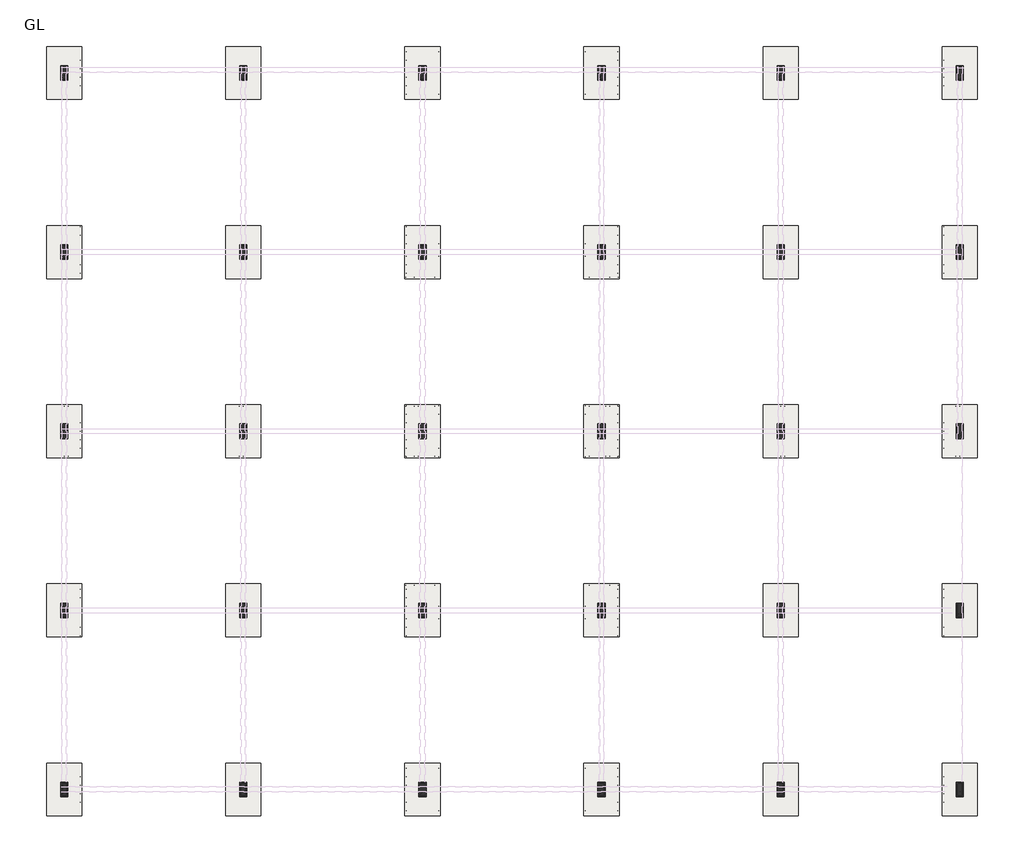
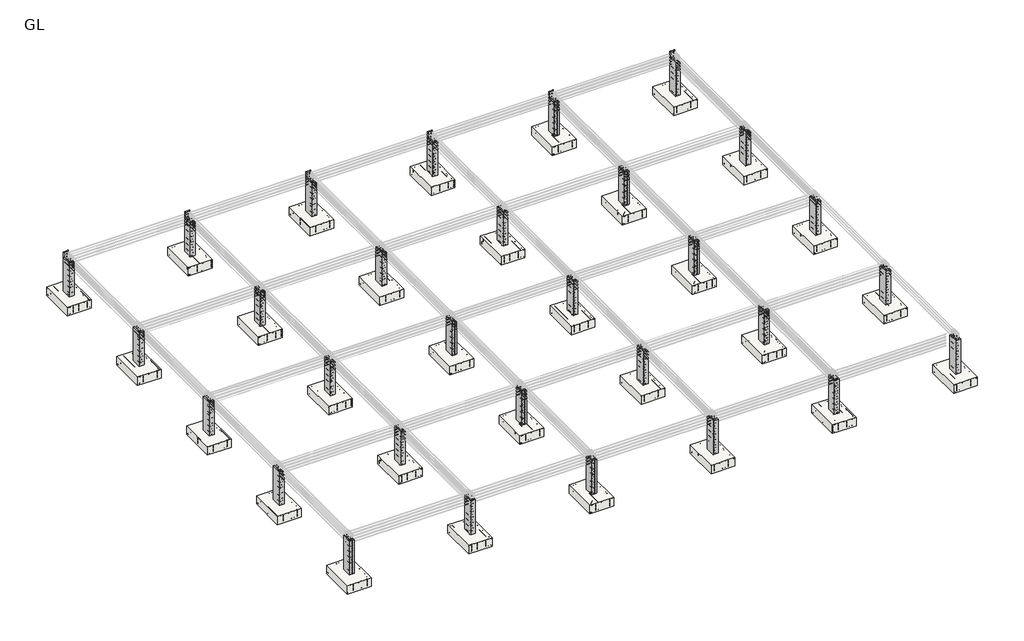
# One storey, part 1 of 16: 30 columns, 30 slabs.
"""IFC4 building model written with IfcOpenShell, lengths in millimetres."""

from ifc_helpers import new_model, si_unit, frame, origin, place, context, project, spatial, polyline, outline, extrude, faceted_brep, element, save

model = new_model("IFC4")

# Units and contexts
model_context = context("Model", 3, world=origin())
ifc_project = project(units=[si_unit("LENGTHUNIT", "METRE", prefix="MILLI")], contexts=[model_context])

# Site, building, storey
site = spatial("IfcSite", under=ifc_project)
building = spatial("IfcBuilding", under=site)
storey = spatial("IfcBuildingStorey", under=building, Name="GL", Elevation=-1829.0)

# Columns
placement = place(None, origin())
element("IfcColumn", 1, ObjectType="Concrete-Rectangular-Column : 500X250", at=placement, inside=storey, context=model_context, shape_type="SweptSolid", body=[
    extrude(outline(polyline([(4354.8832479, -1829.0), (3854.8832479, -1829.0), (3854.8832479, -29.0), (4354.0653602, -29.0), (4354.0653602, 271.0), (4354.8832479, 271.0), (4354.8832479, -1829.0)])), frame((-22931.9544379, 0.0, 0.0), z_axis=(1.0, 0.0, 0.0), x_axis=(0.0, 1.0, 0.0)), (0.0, 0.0, 1.0), 250.0),
])
element("IfcColumn", 2, ObjectType="Concrete-Rectangular-Column : 500X250", at=placement, inside=storey, context=model_context, shape_type="SweptSolid", body=[
    extrude(outline(polyline([(-22681.9544379, -20029.1167521), (-22681.9544379, -20529.1167521), (-22931.9544379, -20529.1167521), (-22931.9544379, -20029.1167521), (-22681.9544379, -20029.1167521)])), frame((0.0, 0.0, -1829.0), z_axis=(0.0, 0.0, 1.0), x_axis=(1.0, 0.0, 0.0)), (0.0, 0.0, 1.0), 1800.0),
])
element("IfcColumn", 3, ObjectType="Concrete-Rectangular-Column : 500X250", at=placement, inside=storey, context=model_context, shape_type="SweptSolid", body=[
    extrude(outline(polyline([(-16585.9544379, -20029.1167521), (-16585.9544379, -20529.1167521), (-16835.9544379, -20529.1167521), (-16835.9544379, -20029.1167521), (-16585.9544379, -20029.1167521)])), frame((0.0, 0.0, -1829.0), z_axis=(0.0, 0.0, 1.0), x_axis=(1.0, 0.0, 0.0)), (0.0, 0.0, 1.0), 1800.0),
])
element("IfcColumn", 4, ObjectType="Concrete-Rectangular-Column : 500X250", at=placement, inside=storey, context=model_context, shape_type="SweptSolid", body=[
    extrude(outline(polyline([(-10489.9544379, -20029.1167521), (-10489.9544379, -20529.1167521), (-10739.9544379, -20529.1167521), (-10739.9544379, -20029.1167521), (-10489.9544379, -20029.1167521)])), frame((0.0, 0.0, -1829.0), z_axis=(0.0, 0.0, 1.0), x_axis=(1.0, 0.0, 0.0)), (0.0, 0.0, 1.0), 1800.0),
])
element("IfcColumn", 5, ObjectType="Concrete-Rectangular-Column : 500X250", at=placement, inside=storey, context=model_context, shape_type="SweptSolid", body=[
    extrude(outline(polyline([(-4393.9544379, -20029.1167521), (-4393.9544379, -20529.1167521), (-4643.9544379, -20529.1167521), (-4643.9544379, -20029.1167521), (-4393.9544379, -20029.1167521)])), frame((0.0, 0.0, -1829.0), z_axis=(0.0, 0.0, 1.0), x_axis=(1.0, 0.0, 0.0)), (0.0, 0.0, 1.0), 1800.0),
])
element("IfcColumn", 6, ObjectType="Concrete-Rectangular-Column : 500X250", at=placement, inside=storey, context=model_context, shape_type="SweptSolid", body=[
    extrude(outline(polyline([(1702.0455621, -20029.1167521), (1702.0455621, -20529.1167521), (1452.0455621, -20529.1167521), (1452.0455621, -20029.1167521), (1702.0455621, -20029.1167521)])), frame((0.0, 0.0, -1829.0), z_axis=(0.0, 0.0, 1.0), x_axis=(1.0, 0.0, 0.0)), (0.0, 0.0, 1.0), 1800.0),
])
element("IfcColumn", 7, ObjectType="Concrete-Rectangular-Column : 500X250", at=placement, inside=storey, context=model_context, shape_type="SweptSolid", body=[
    extrude(outline(polyline([(7798.0455621, -20029.1167521), (7798.0455621, -20529.1167521), (7548.0455621, -20529.1167521), (7548.0455621, -20029.1167521), (7798.0455621, -20029.1167521)])), frame((0.0, 0.0, -1829.0), z_axis=(0.0, 0.0, 1.0), x_axis=(1.0, 0.0, 0.0)), (0.0, 0.0, 1.0), 1800.0),
])
element("IfcColumn", 8, ObjectType="Concrete-Rectangular-Column : 500X250", at=placement, inside=storey, context=model_context, shape_type="SweptSolid", body=[
    extrude(outline(polyline([(-22681.9544379, -13933.1167521), (-22681.9544379, -14433.1167521), (-22931.9544379, -14433.1167521), (-22931.9544379, -13933.1167521), (-22681.9544379, -13933.1167521)])), frame((0.0, 0.0, -1829.0), z_axis=(0.0, 0.0, 1.0), x_axis=(1.0, 0.0, 0.0)), (0.0, 0.0, 1.0), 1800.0),
])
element("IfcColumn", 9, ObjectType="Concrete-Rectangular-Column : 500X250", at=placement, inside=storey, context=model_context, shape_type="SweptSolid", body=[
    extrude(outline(polyline([(-16585.9544379, -13933.1167521), (-16585.9544379, -14433.1167521), (-16835.9544379, -14433.1167521), (-16835.9544379, -13933.1167521), (-16585.9544379, -13933.1167521)])), frame((0.0, 0.0, -1829.0), z_axis=(0.0, 0.0, 1.0), x_axis=(1.0, 0.0, 0.0)), (0.0, 0.0, 1.0), 1800.0),
])
element("IfcColumn", 10, ObjectType="Concrete-Rectangular-Column : 500X250", at=placement, inside=storey, context=model_context, shape_type="SweptSolid", body=[
    extrude(outline(polyline([(-10489.9544379, -13933.1167521), (-10489.9544379, -14433.1167521), (-10739.9544379, -14433.1167521), (-10739.9544379, -13933.1167521), (-10489.9544379, -13933.1167521)])), frame((0.0, 0.0, -1829.0), z_axis=(0.0, 0.0, 1.0), x_axis=(1.0, 0.0, 0.0)), (0.0, 0.0, 1.0), 1800.0),
])
element("IfcColumn", 11, ObjectType="Concrete-Rectangular-Column : 500X250", at=placement, inside=storey, context=model_context, shape_type="SweptSolid", body=[
    extrude(outline(polyline([(-4393.9544379, -13933.1167521), (-4393.9544379, -14433.1167521), (-4643.9544379, -14433.1167521), (-4643.9544379, -13933.1167521), (-4393.9544379, -13933.1167521)])), frame((0.0, 0.0, -1829.0), z_axis=(0.0, 0.0, 1.0), x_axis=(1.0, 0.0, 0.0)), (0.0, 0.0, 1.0), 1800.0),
])
element("IfcColumn", 12, ObjectType="Concrete-Rectangular-Column : 500X250", at=placement, inside=storey, context=model_context, shape_type="SweptSolid", body=[
    extrude(outline(polyline([(1702.0455621, -13933.1167521), (1702.0455621, -14433.1167521), (1452.0455621, -14433.1167521), (1452.0455621, -13933.1167521), (1702.0455621, -13933.1167521)])), frame((0.0, 0.0, -1829.0), z_axis=(0.0, 0.0, 1.0), x_axis=(1.0, 0.0, 0.0)), (0.0, 0.0, 1.0), 1800.0),
])
element("IfcColumn", 13, ObjectType="Concrete-Rectangular-Column : 500X250", at=placement, inside=storey, context=model_context, shape_type="SweptSolid", body=[
    extrude(outline(polyline([(7798.0455621, -13933.1167521), (7798.0455621, -14433.1167521), (7548.0455621, -14433.1167521), (7548.0455621, -13933.1167521), (7798.0455621, -13933.1167521)])), frame((0.0, 0.0, -1829.0), z_axis=(0.0, 0.0, 1.0), x_axis=(1.0, 0.0, 0.0)), (0.0, 0.0, 1.0), 1800.0),
])
element("IfcColumn", 14, ObjectType="Concrete-Rectangular-Column : 500X250", at=placement, inside=storey, context=model_context, shape_type="SweptSolid", body=[
    extrude(outline(polyline([(-22681.9544379, -7837.1167521), (-22681.9544379, -8337.1167521), (-22931.9544379, -8337.1167521), (-22931.9544379, -7837.1167521), (-22681.9544379, -7837.1167521)])), frame((0.0, 0.0, -1829.0), z_axis=(0.0, 0.0, 1.0), x_axis=(1.0, 0.0, 0.0)), (0.0, 0.0, 1.0), 1800.0),
])
element("IfcColumn", 15, ObjectType="Concrete-Rectangular-Column : 500X250", at=placement, inside=storey, context=model_context, shape_type="SweptSolid", body=[
    extrude(outline(polyline([(-16585.9544379, -7837.1167521), (-16585.9544379, -8337.1167521), (-16835.9544379, -8337.1167521), (-16835.9544379, -7837.1167521), (-16585.9544379, -7837.1167521)])), frame((0.0, 0.0, -1829.0), z_axis=(0.0, 0.0, 1.0), x_axis=(1.0, 0.0, 0.0)), (0.0, 0.0, 1.0), 1800.0),
])
element("IfcColumn", 16, ObjectType="Concrete-Rectangular-Column : 500X250", at=placement, inside=storey, context=model_context, shape_type="SweptSolid", body=[
    extrude(outline(polyline([(-10489.9544379, -7837.1167521), (-10489.9544379, -8337.1167521), (-10739.9544379, -8337.1167521), (-10739.9544379, -7837.1167521), (-10489.9544379, -7837.1167521)])), frame((0.0, 0.0, -1829.0), z_axis=(0.0, 0.0, 1.0), x_axis=(1.0, 0.0, 0.0)), (0.0, 0.0, 1.0), 1800.0),
])
element("IfcColumn", 17, ObjectType="Concrete-Rectangular-Column : 500X250", at=placement, inside=storey, context=model_context, shape_type="SweptSolid", body=[
    extrude(outline(polyline([(-4393.9544379, -7837.1167521), (-4393.9544379, -8337.1167521), (-4643.9544379, -8337.1167521), (-4643.9544379, -7837.1167521), (-4393.9544379, -7837.1167521)])), frame((0.0, 0.0, -1829.0), z_axis=(0.0, 0.0, 1.0), x_axis=(1.0, 0.0, 0.0)), (0.0, 0.0, 1.0), 1800.0),
])
element("IfcColumn", 18, ObjectType="Concrete-Rectangular-Column : 500X250", at=placement, inside=storey, context=model_context, shape_type="SweptSolid", body=[
    extrude(outline(polyline([(1702.0455621, -7837.1167521), (1702.0455621, -8337.1167521), (1452.0455621, -8337.1167521), (1452.0455621, -7837.1167521), (1702.0455621, -7837.1167521)])), frame((0.0, 0.0, -1829.0), z_axis=(0.0, 0.0, 1.0), x_axis=(1.0, 0.0, 0.0)), (0.0, 0.0, 1.0), 1800.0),
])
element("IfcColumn", 19, ObjectType="Concrete-Rectangular-Column : 500X250", at=placement, inside=storey, context=model_context, shape_type="SweptSolid", body=[
    extrude(outline(polyline([(7798.0455621, -7837.1167521), (7798.0455621, -8337.1167521), (7548.0455621, -8337.1167521), (7548.0455621, -7837.1167521), (7798.0455621, -7837.1167521)])), frame((0.0, 0.0, -1829.0), z_axis=(0.0, 0.0, 1.0), x_axis=(1.0, 0.0, 0.0)), (0.0, 0.0, 1.0), 1800.0),
])
element("IfcColumn", 20, ObjectType="Concrete-Rectangular-Column : 500X250", at=placement, inside=storey, context=model_context, shape_type="SweptSolid", body=[
    extrude(outline(polyline([(-22681.9544379, -1741.1167521), (-22681.9544379, -2241.1167521), (-22931.9544379, -2241.1167521), (-22931.9544379, -1741.1167521), (-22681.9544379, -1741.1167521)])), frame((0.0, 0.0, -1829.0), z_axis=(0.0, 0.0, 1.0), x_axis=(1.0, 0.0, 0.0)), (0.0, 0.0, 1.0), 1800.0),
])
element("IfcColumn", 21, ObjectType="Concrete-Rectangular-Column : 500X250", at=placement, inside=storey, context=model_context, shape_type="SweptSolid", body=[
    extrude(outline(polyline([(-16585.9544379, -1741.1167521), (-16585.9544379, -2241.1167521), (-16835.9544379, -2241.1167521), (-16835.9544379, -1741.1167521), (-16585.9544379, -1741.1167521)])), frame((0.0, 0.0, -1829.0), z_axis=(0.0, 0.0, 1.0), x_axis=(1.0, 0.0, 0.0)), (0.0, 0.0, 1.0), 1800.0),
])
element("IfcColumn", 22, ObjectType="Concrete-Rectangular-Column : 500X250", at=placement, inside=storey, context=model_context, shape_type="SweptSolid", body=[
    extrude(outline(polyline([(-10489.9544379, -1741.1167521), (-10489.9544379, -2241.1167521), (-10739.9544379, -2241.1167521), (-10739.9544379, -1741.1167521), (-10489.9544379, -1741.1167521)])), frame((0.0, 0.0, -1829.0), z_axis=(0.0, 0.0, 1.0), x_axis=(1.0, 0.0, 0.0)), (0.0, 0.0, 1.0), 1800.0),
])
element("IfcColumn", 23, ObjectType="Concrete-Rectangular-Column : 500X250", at=placement, inside=storey, context=model_context, shape_type="SweptSolid", body=[
    extrude(outline(polyline([(-4393.9544379, -1741.1167521), (-4393.9544379, -2241.1167521), (-4643.9544379, -2241.1167521), (-4643.9544379, -1741.1167521), (-4393.9544379, -1741.1167521)])), frame((0.0, 0.0, -1829.0), z_axis=(0.0, 0.0, 1.0), x_axis=(1.0, 0.0, 0.0)), (0.0, 0.0, 1.0), 1800.0),
])
element("IfcColumn", 24, ObjectType="Concrete-Rectangular-Column : 500X250", at=placement, inside=storey, context=model_context, shape_type="SweptSolid", body=[
    extrude(outline(polyline([(1702.0455621, -1741.1167521), (1702.0455621, -2241.1167521), (1452.0455621, -2241.1167521), (1452.0455621, -1741.1167521), (1702.0455621, -1741.1167521)])), frame((0.0, 0.0, -1829.0), z_axis=(0.0, 0.0, 1.0), x_axis=(1.0, 0.0, 0.0)), (0.0, 0.0, 1.0), 1800.0),
])
element("IfcColumn", 25, ObjectType="Concrete-Rectangular-Column : 500X250", at=placement, inside=storey, context=model_context, shape_type="SweptSolid", body=[
    extrude(outline(polyline([(7798.0455621, -1741.1167521), (7798.0455621, -2241.1167521), (7548.0455621, -2241.1167521), (7548.0455621, -1741.1167521), (7798.0455621, -1741.1167521)])), frame((0.0, 0.0, -1829.0), z_axis=(0.0, 0.0, 1.0), x_axis=(1.0, 0.0, 0.0)), (0.0, 0.0, 1.0), 1800.0),
])
element("IfcColumn", 26, ObjectType="Concrete-Rectangular-Column : 500X250", at=placement, inside=storey, context=model_context, shape_type="Brep", body=[
    faceted_brep([(-16585.9544379, 4354.8832479, 271.0), (-16835.9544379, 4354.8832479, 271.0), (-16835.9544379, 4354.0653602, 271.0), (-16585.9544379, 4354.0653602, 271.0), (-16585.9544379, 4354.8832479, -1829.0), (-16585.9544379, 3854.8832479, -1829.0), (-16835.9544379, 3854.8832479, -1829.0), (-16835.9544379, 4354.8832479, -1829.0), (-16835.9544379, 3854.8832479, -29.0), (-16835.9544379, 4054.0653602, -29.0), (-16835.9544379, 4354.0653602, -29.0), (-16585.9544379, 3854.8832479, -29.0), (-16585.9544379, 4354.0653602, -29.0), (-16585.9544379, 4054.0653602, -29.0)], [[[0, 1, 2, 3]], [[4, 5, 6, 7]], [[1, 0, 4, 7]], [[7, 6, 8, 9, 10, 2, 1]], [[6, 5, 11, 8]], [[5, 4, 0, 3, 12, 13, 11]], [[12, 10, 9, 8, 11, 13]], [[10, 12, 3, 2]]]),
])
element("IfcColumn", 27, ObjectType="Concrete-Rectangular-Column : 500X250", at=placement, inside=storey, context=model_context, shape_type="Brep", body=[
    faceted_brep([(-10489.9544379, 4354.8832479, 271.0), (-10739.9544379, 4354.8832479, 271.0), (-10739.9544379, 4354.0653602, 271.0), (-10489.9544379, 4354.0653602, 271.0), (-10489.9544379, 4354.8832479, -1829.0), (-10489.9544379, 3854.8832479, -1829.0), (-10739.9544379, 3854.8832479, -1829.0), (-10739.9544379, 4354.8832479, -1829.0), (-10739.9544379, 3854.8832479, -29.0), (-10739.9544379, 4054.0653602, -29.0), (-10739.9544379, 4354.0653602, -29.0), (-10489.9544379, 3854.8832479, -29.0), (-10489.9544379, 4354.0653602, -29.0), (-10489.9544379, 4054.0653602, -29.0)], [[[0, 1, 2, 3]], [[4, 5, 6, 7]], [[1, 0, 4, 7]], [[7, 6, 8, 9, 10, 2, 1]], [[6, 5, 11, 8]], [[5, 4, 0, 3, 12, 13, 11]], [[12, 10, 9, 8, 11, 13]], [[10, 12, 3, 2]]]),
])
element("IfcColumn", 28, ObjectType="Concrete-Rectangular-Column : 500X250", at=placement, inside=storey, context=model_context, shape_type="Brep", body=[
    faceted_brep([(-4393.9544379, 4354.8832479, 271.0), (-4643.9544379, 4354.8832479, 271.0), (-4643.9544379, 4354.0653602, 271.0), (-4393.9544379, 4354.0653602, 271.0), (-4393.9544379, 4354.8832479, -1829.0), (-4393.9544379, 3854.8832479, -1829.0), (-4643.9544379, 3854.8832479, -1829.0), (-4643.9544379, 4354.8832479, -1829.0), (-4643.9544379, 3854.8832479, -29.0), (-4643.9544379, 4054.0653602, -29.0), (-4643.9544379, 4354.0653602, -29.0), (-4393.9544379, 3854.8832479, -29.0), (-4393.9544379, 4354.0653602, -29.0), (-4393.9544379, 4054.0653602, -29.0)], [[[0, 1, 2, 3]], [[4, 5, 6, 7]], [[1, 0, 4, 7]], [[7, 6, 8, 9, 10, 2, 1]], [[6, 5, 11, 8]], [[5, 4, 0, 3, 12, 13, 11]], [[12, 10, 9, 8, 11, 13]], [[10, 12, 3, 2]]]),
])
element("IfcColumn", 29, ObjectType="Concrete-Rectangular-Column : 500X250", at=placement, inside=storey, context=model_context, shape_type="Brep", body=[
    faceted_brep([(1702.0455621, 4354.8832479, 271.0), (1452.0455621, 4354.8832479, 271.0), (1452.0455621, 4354.0653602, 271.0), (1702.0455621, 4354.0653602, 271.0), (1702.0455621, 4354.8832479, -1829.0), (1702.0455621, 3854.8832479, -1829.0), (1452.0455621, 3854.8832479, -1829.0), (1452.0455621, 4354.8832479, -1829.0), (1452.0455621, 3854.8832479, -29.0), (1452.0455621, 4054.0653602, -29.0), (1452.0455621, 4354.0653602, -29.0), (1702.0455621, 3854.8832479, -29.0), (1702.0455621, 4354.0653602, -29.0), (1702.0455621, 4054.0653602, -29.0)], [[[0, 1, 2, 3]], [[4, 5, 6, 7]], [[1, 0, 4, 7]], [[7, 6, 8, 9, 10, 2, 1]], [[6, 5, 11, 8]], [[5, 4, 0, 3, 12, 13, 11]], [[12, 10, 9, 8, 11, 13]], [[10, 12, 3, 2]]]),
])
element("IfcColumn", 30, ObjectType="Concrete-Rectangular-Column : 500X250", at=placement, inside=storey, context=model_context, shape_type="SweptSolid", body=[
    extrude(outline(polyline([(4354.8832479, -1829.0), (3854.8832479, -1829.0), (3854.8832479, -29.0), (4354.0653602, -29.0), (4354.0653602, 271.0), (4354.8832479, 271.0), (4354.8832479, -1829.0)])), frame((7548.0455621, 0.0, 0.0), z_axis=(1.0, 0.0, 0.0), x_axis=(0.0, 1.0, 0.0)), (0.0, 0.0, 1.0), 250.0),
])

# Slabs
element("IfcSlab", 31, ObjectType="Footing-Rectangular : 1800 x 1200 x 450mm", at=placement, inside=storey, context=model_context, shape_type="SweptSolid", body=[
    extrude(outline(polyline([(-22206.9544379, 5004.8832479), (-22206.9544379, 3204.8832479), (-23406.9544379, 3204.8832479), (-23406.9544379, 5004.8832479), (-22206.9544379, 5004.8832479)])), frame((0.0, 0.0, -2279.0), z_axis=(0.0, 0.0, 1.0), x_axis=(1.0, 0.0, 0.0)), (0.0, 0.0, 1.0), 450.0),
])
element("IfcSlab", 32, ObjectType="Footing-Rectangular : 1800 x 1200 x 450mm", at=placement, inside=storey, context=model_context, shape_type="SweptSolid", body=[
    extrude(outline(polyline([(-22206.9544379, -19379.1167521), (-22206.9544379, -21179.1167521), (-23406.9544379, -21179.1167521), (-23406.9544379, -19379.1167521), (-22206.9544379, -19379.1167521)])), frame((0.0, 0.0, -2279.0), z_axis=(0.0, 0.0, 1.0), x_axis=(1.0, 0.0, 0.0)), (0.0, 0.0, 1.0), 450.0),
])
element("IfcSlab", 33, ObjectType="Footing-Rectangular : 1800 x 1200 x 450mm", at=placement, inside=storey, context=model_context, shape_type="SweptSolid", body=[
    extrude(outline(polyline([(-16110.9544379, -19379.1167521), (-16110.9544379, -21179.1167521), (-17310.9544379, -21179.1167521), (-17310.9544379, -19379.1167521), (-16110.9544379, -19379.1167521)])), frame((0.0, 0.0, -2279.0), z_axis=(0.0, 0.0, 1.0), x_axis=(1.0, 0.0, 0.0)), (0.0, 0.0, 1.0), 450.0),
])
element("IfcSlab", 34, ObjectType="Footing-Rectangular : 1800 x 1200 x 450mm", at=placement, inside=storey, context=model_context, shape_type="SweptSolid", body=[
    extrude(outline(polyline([(-10014.9544379, -19379.1167521), (-10014.9544379, -21179.1167521), (-11214.9544379, -21179.1167521), (-11214.9544379, -19379.1167521), (-10014.9544379, -19379.1167521)])), frame((0.0, 0.0, -2279.0), z_axis=(0.0, 0.0, 1.0), x_axis=(1.0, 0.0, 0.0)), (0.0, 0.0, 1.0), 450.0),
])
element("IfcSlab", 35, ObjectType="Footing-Rectangular : 1800 x 1200 x 450mm", at=placement, inside=storey, context=model_context, shape_type="SweptSolid", body=[
    extrude(outline(polyline([(-3918.9544379, -19379.1167521), (-3918.9544379, -21179.1167521), (-5118.9544379, -21179.1167521), (-5118.9544379, -19379.1167521), (-3918.9544379, -19379.1167521)])), frame((0.0, 0.0, -2279.0), z_axis=(0.0, 0.0, 1.0), x_axis=(1.0, 0.0, 0.0)), (0.0, 0.0, 1.0), 450.0),
])
element("IfcSlab", 36, ObjectType="Footing-Rectangular : 1800 x 1200 x 450mm", at=placement, inside=storey, context=model_context, shape_type="SweptSolid", body=[
    extrude(outline(polyline([(2177.0455621, -19379.1167521), (2177.0455621, -21179.1167521), (977.0455621, -21179.1167521), (977.0455621, -19379.1167521), (2177.0455621, -19379.1167521)])), frame((0.0, 0.0, -2279.0), z_axis=(0.0, 0.0, 1.0), x_axis=(1.0, 0.0, 0.0)), (0.0, 0.0, 1.0), 450.0),
])
element("IfcSlab", 37, ObjectType="Footing-Rectangular : 1800 x 1200 x 450mm", at=placement, inside=storey, context=model_context, shape_type="SweptSolid", body=[
    extrude(outline(polyline([(8273.0455621, -19379.1167521), (8273.0455621, -21179.1167521), (7073.0455621, -21179.1167521), (7073.0455621, -19379.1167521), (8273.0455621, -19379.1167521)])), frame((0.0, 0.0, -2279.0), z_axis=(0.0, 0.0, 1.0), x_axis=(1.0, 0.0, 0.0)), (0.0, 0.0, 1.0), 450.0),
])
element("IfcSlab", 38, ObjectType="Footing-Rectangular : 1800 x 1200 x 450mm", at=placement, inside=storey, context=model_context, shape_type="SweptSolid", body=[
    extrude(outline(polyline([(-22206.9544379, -13283.1167521), (-22206.9544379, -15083.1167521), (-23406.9544379, -15083.1167521), (-23406.9544379, -13283.1167521), (-22206.9544379, -13283.1167521)])), frame((0.0, 0.0, -2279.0), z_axis=(0.0, 0.0, 1.0), x_axis=(1.0, 0.0, 0.0)), (0.0, 0.0, 1.0), 450.0),
])
element("IfcSlab", 39, ObjectType="Footing-Rectangular : 1800 x 1200 x 450mm", at=placement, inside=storey, context=model_context, shape_type="SweptSolid", body=[
    extrude(outline(polyline([(-16110.9544379, -13283.1167521), (-16110.9544379, -15083.1167521), (-17310.9544379, -15083.1167521), (-17310.9544379, -13283.1167521), (-16110.9544379, -13283.1167521)])), frame((0.0, 0.0, -2279.0), z_axis=(0.0, 0.0, 1.0), x_axis=(1.0, 0.0, 0.0)), (0.0, 0.0, 1.0), 450.0),
])
element("IfcSlab", 40, ObjectType="Footing-Rectangular : 1800 x 1200 x 450mm", at=placement, inside=storey, context=model_context, shape_type="SweptSolid", body=[
    extrude(outline(polyline([(-10014.9544379, -13283.1167521), (-10014.9544379, -15083.1167521), (-11214.9544379, -15083.1167521), (-11214.9544379, -13283.1167521), (-10014.9544379, -13283.1167521)])), frame((0.0, 0.0, -2279.0), z_axis=(0.0, 0.0, 1.0), x_axis=(1.0, 0.0, 0.0)), (0.0, 0.0, 1.0), 450.0),
])
element("IfcSlab", 41, ObjectType="Footing-Rectangular : 1800 x 1200 x 450mm", at=placement, inside=storey, context=model_context, shape_type="SweptSolid", body=[
    extrude(outline(polyline([(-3918.9544379, -13283.1167521), (-3918.9544379, -15083.1167521), (-5118.9544379, -15083.1167521), (-5118.9544379, -13283.1167521), (-3918.9544379, -13283.1167521)])), frame((0.0, 0.0, -2279.0), z_axis=(0.0, 0.0, 1.0), x_axis=(1.0, 0.0, 0.0)), (0.0, 0.0, 1.0), 450.0),
])
element("IfcSlab", 42, ObjectType="Footing-Rectangular : 1800 x 1200 x 450mm", at=placement, inside=storey, context=model_context, shape_type="SweptSolid", body=[
    extrude(outline(polyline([(2177.0455621, -13283.1167521), (2177.0455621, -15083.1167521), (977.0455621, -15083.1167521), (977.0455621, -13283.1167521), (2177.0455621, -13283.1167521)])), frame((0.0, 0.0, -2279.0), z_axis=(0.0, 0.0, 1.0), x_axis=(1.0, 0.0, 0.0)), (0.0, 0.0, 1.0), 450.0),
])
element("IfcSlab", 43, ObjectType="Footing-Rectangular : 1800 x 1200 x 450mm", at=placement, inside=storey, context=model_context, shape_type="SweptSolid", body=[
    extrude(outline(polyline([(8273.0455621, -13283.1167521), (8273.0455621, -15083.1167521), (7073.0455621, -15083.1167521), (7073.0455621, -13283.1167521), (8273.0455621, -13283.1167521)])), frame((0.0, 0.0, -2279.0), z_axis=(0.0, 0.0, 1.0), x_axis=(1.0, 0.0, 0.0)), (0.0, 0.0, 1.0), 450.0),
])
element("IfcSlab", 44, ObjectType="Footing-Rectangular : 1800 x 1200 x 450mm", at=placement, inside=storey, context=model_context, shape_type="SweptSolid", body=[
    extrude(outline(polyline([(-22206.9544379, -7187.1167521), (-22206.9544379, -8987.1167521), (-23406.9544379, -8987.1167521), (-23406.9544379, -7187.1167521), (-22206.9544379, -7187.1167521)])), frame((0.0, 0.0, -2279.0), z_axis=(0.0, 0.0, 1.0), x_axis=(1.0, 0.0, 0.0)), (0.0, 0.0, 1.0), 450.0),
])
element("IfcSlab", 45, ObjectType="Footing-Rectangular : 1800 x 1200 x 450mm", at=placement, inside=storey, context=model_context, shape_type="SweptSolid", body=[
    extrude(outline(polyline([(-16110.9544379, -7187.1167521), (-16110.9544379, -8987.1167521), (-17310.9544379, -8987.1167521), (-17310.9544379, -7187.1167521), (-16110.9544379, -7187.1167521)])), frame((0.0, 0.0, -2279.0), z_axis=(0.0, 0.0, 1.0), x_axis=(1.0, 0.0, 0.0)), (0.0, 0.0, 1.0), 450.0),
])
element("IfcSlab", 46, ObjectType="Footing-Rectangular : 1800 x 1200 x 450mm", at=placement, inside=storey, context=model_context, shape_type="SweptSolid", body=[
    extrude(outline(polyline([(-10014.9544379, -7187.1167521), (-10014.9544379, -8987.1167521), (-11214.9544379, -8987.1167521), (-11214.9544379, -7187.1167521), (-10014.9544379, -7187.1167521)])), frame((0.0, 0.0, -2279.0), z_axis=(0.0, 0.0, 1.0), x_axis=(1.0, 0.0, 0.0)), (0.0, 0.0, 1.0), 450.0),
])
element("IfcSlab", 47, ObjectType="Footing-Rectangular : 1800 x 1200 x 450mm", at=placement, inside=storey, context=model_context, shape_type="SweptSolid", body=[
    extrude(outline(polyline([(-3918.9544379, -7187.1167521), (-3918.9544379, -8987.1167521), (-5118.9544379, -8987.1167521), (-5118.9544379, -7187.1167521), (-3918.9544379, -7187.1167521)])), frame((0.0, 0.0, -2279.0), z_axis=(0.0, 0.0, 1.0), x_axis=(1.0, 0.0, 0.0)), (0.0, 0.0, 1.0), 450.0),
])
element("IfcSlab", 48, ObjectType="Footing-Rectangular : 1800 x 1200 x 450mm", at=placement, inside=storey, context=model_context, shape_type="SweptSolid", body=[
    extrude(outline(polyline([(2177.0455621, -7187.1167521), (2177.0455621, -8987.1167521), (977.0455621, -8987.1167521), (977.0455621, -7187.1167521), (2177.0455621, -7187.1167521)])), frame((0.0, 0.0, -2279.0), z_axis=(0.0, 0.0, 1.0), x_axis=(1.0, 0.0, 0.0)), (0.0, 0.0, 1.0), 450.0),
])
element("IfcSlab", 49, ObjectType="Footing-Rectangular : 1800 x 1200 x 450mm", at=placement, inside=storey, context=model_context, shape_type="SweptSolid", body=[
    extrude(outline(polyline([(8273.0455621, -7187.1167521), (8273.0455621, -8987.1167521), (7073.0455621, -8987.1167521), (7073.0455621, -7187.1167521), (8273.0455621, -7187.1167521)])), frame((0.0, 0.0, -2279.0), z_axis=(0.0, 0.0, 1.0), x_axis=(1.0, 0.0, 0.0)), (0.0, 0.0, 1.0), 450.0),
])
element("IfcSlab", 50, ObjectType="Footing-Rectangular : 1800 x 1200 x 450mm", at=placement, inside=storey, context=model_context, shape_type="SweptSolid", body=[
    extrude(outline(polyline([(-22206.9544379, -1091.1167521), (-22206.9544379, -2891.1167521), (-23406.9544379, -2891.1167521), (-23406.9544379, -1091.1167521), (-22206.9544379, -1091.1167521)])), frame((0.0, 0.0, -2279.0), z_axis=(0.0, 0.0, 1.0), x_axis=(1.0, 0.0, 0.0)), (0.0, 0.0, 1.0), 450.0),
])
element("IfcSlab", 51, ObjectType="Footing-Rectangular : 1800 x 1200 x 450mm", at=placement, inside=storey, context=model_context, shape_type="SweptSolid", body=[
    extrude(outline(polyline([(-16110.9544379, -1091.1167521), (-16110.9544379, -2891.1167521), (-17310.9544379, -2891.1167521), (-17310.9544379, -1091.1167521), (-16110.9544379, -1091.1167521)])), frame((0.0, 0.0, -2279.0), z_axis=(0.0, 0.0, 1.0), x_axis=(1.0, 0.0, 0.0)), (0.0, 0.0, 1.0), 450.0),
])
element("IfcSlab", 52, ObjectType="Footing-Rectangular : 1800 x 1200 x 450mm", at=placement, inside=storey, context=model_context, shape_type="SweptSolid", body=[
    extrude(outline(polyline([(-10014.9544379, -1091.1167521), (-10014.9544379, -2891.1167521), (-11214.9544379, -2891.1167521), (-11214.9544379, -1091.1167521), (-10014.9544379, -1091.1167521)])), frame((0.0, 0.0, -2279.0), z_axis=(0.0, 0.0, 1.0), x_axis=(1.0, 0.0, 0.0)), (0.0, 0.0, 1.0), 450.0),
])
element("IfcSlab", 53, ObjectType="Footing-Rectangular : 1800 x 1200 x 450mm", at=placement, inside=storey, context=model_context, shape_type="SweptSolid", body=[
    extrude(outline(polyline([(-3918.9544379, -1091.1167521), (-3918.9544379, -2891.1167521), (-5118.9544379, -2891.1167521), (-5118.9544379, -1091.1167521), (-3918.9544379, -1091.1167521)])), frame((0.0, 0.0, -2279.0), z_axis=(0.0, 0.0, 1.0), x_axis=(1.0, 0.0, 0.0)), (0.0, 0.0, 1.0), 450.0),
])
element("IfcSlab", 54, ObjectType="Footing-Rectangular : 1800 x 1200 x 450mm", at=placement, inside=storey, context=model_context, shape_type="SweptSolid", body=[
    extrude(outline(polyline([(2177.0455621, -1091.1167521), (2177.0455621, -2891.1167521), (977.0455621, -2891.1167521), (977.0455621, -1091.1167521), (2177.0455621, -1091.1167521)])), frame((0.0, 0.0, -2279.0), z_axis=(0.0, 0.0, 1.0), x_axis=(1.0, 0.0, 0.0)), (0.0, 0.0, 1.0), 450.0),
])
element("IfcSlab", 55, ObjectType="Footing-Rectangular : 1800 x 1200 x 450mm", at=placement, inside=storey, context=model_context, shape_type="SweptSolid", body=[
    extrude(outline(polyline([(8273.0455621, -1091.1167521), (8273.0455621, -2891.1167521), (7073.0455621, -2891.1167521), (7073.0455621, -1091.1167521), (8273.0455621, -1091.1167521)])), frame((0.0, 0.0, -2279.0), z_axis=(0.0, 0.0, 1.0), x_axis=(1.0, 0.0, 0.0)), (0.0, 0.0, 1.0), 450.0),
])
element("IfcSlab", 56, ObjectType="Footing-Rectangular : 1800 x 1200 x 450mm", at=placement, inside=storey, context=model_context, shape_type="SweptSolid", body=[
    extrude(outline(polyline([(-16110.9544379, 5004.8832479), (-16110.9544379, 3204.8832479), (-17310.9544379, 3204.8832479), (-17310.9544379, 5004.8832479), (-16110.9544379, 5004.8832479)])), frame((0.0, 0.0, -2279.0), z_axis=(0.0, 0.0, 1.0), x_axis=(1.0, 0.0, 0.0)), (0.0, 0.0, 1.0), 450.0),
])
element("IfcSlab", 57, ObjectType="Footing-Rectangular : 1800 x 1200 x 450mm", at=placement, inside=storey, context=model_context, shape_type="SweptSolid", body=[
    extrude(outline(polyline([(-10014.9544379, 5004.8832479), (-10014.9544379, 3204.8832479), (-11214.9544379, 3204.8832479), (-11214.9544379, 5004.8832479), (-10014.9544379, 5004.8832479)])), frame((0.0, 0.0, -2279.0), z_axis=(0.0, 0.0, 1.0), x_axis=(1.0, 0.0, 0.0)), (0.0, 0.0, 1.0), 450.0),
])
element("IfcSlab", 58, ObjectType="Footing-Rectangular : 1800 x 1200 x 450mm", at=placement, inside=storey, context=model_context, shape_type="SweptSolid", body=[
    extrude(outline(polyline([(-3918.9544379, 5004.8832479), (-3918.9544379, 3204.8832479), (-5118.9544379, 3204.8832479), (-5118.9544379, 5004.8832479), (-3918.9544379, 5004.8832479)])), frame((0.0, 0.0, -2279.0), z_axis=(0.0, 0.0, 1.0), x_axis=(1.0, 0.0, 0.0)), (0.0, 0.0, 1.0), 450.0),
])
element("IfcSlab", 59, ObjectType="Footing-Rectangular : 1800 x 1200 x 450mm", at=placement, inside=storey, context=model_context, shape_type="SweptSolid", body=[
    extrude(outline(polyline([(2177.0455621, 5004.8832479), (2177.0455621, 3204.8832479), (977.0455621, 3204.8832479), (977.0455621, 5004.8832479), (2177.0455621, 5004.8832479)])), frame((0.0, 0.0, -2279.0), z_axis=(0.0, 0.0, 1.0), x_axis=(1.0, 0.0, 0.0)), (0.0, 0.0, 1.0), 450.0),
])
element("IfcSlab", 60, ObjectType="Footing-Rectangular : 1800 x 1200 x 450mm", at=placement, inside=storey, context=model_context, shape_type="SweptSolid", body=[
    extrude(outline(polyline([(8273.0455621, 5004.8832479), (8273.0455621, 3204.8832479), (7073.0455621, 3204.8832479), (7073.0455621, 5004.8832479), (8273.0455621, 5004.8832479)])), frame((0.0, 0.0, -2279.0), z_axis=(0.0, 0.0, 1.0), x_axis=(1.0, 0.0, 0.0)), (0.0, 0.0, 1.0), 450.0),
])

save(model, "model.ifc")

# Revit data of these elements
# Grids (mm)
#   "1": line (13887.362, -20279.117) -> (-30807.258, -20279.117)
#   "2": line (13887.362, -14183.117) -> (-30807.258, -14183.117)
#   "3": line (13887.362, -8087.117) -> (-30807.258, -8087.117)
#   "4": line (13887.362, -1991.117) -> (-30807.258, -1991.117)
#   "5": line (13887.362, 4104.883) -> (-30807.258, 4104.883)
#   "6": line (-22806.954, 9422.959) -> (-22806.954, -33706.633)
#   "7": line (-16710.954, 9422.959) -> (-16710.954, -33706.633)
#   "8": line (-10614.954, 9422.959) -> (-10614.954, -33706.633)
#   "9": line (-4518.954, 9422.959) -> (-4518.954, -33706.633)
#   "10": line (1577.046, 9422.959) -> (1577.046, -33706.633)
#   "11": line (7673.046, 9422.959) -> (7673.046, -33706.633)
#   "12": line (-1859902.039, -3445816.125) -> (-1729902.039, -3445816.125)
# Type "Concrete-Rectangular-Column : 500X250"
#   b = 0' - 9.84252"
#   h = 1' - 7.68504"
#   Structural Material [instance default] = Concrete, Cast-in-Place gray
# Type "Footing-Rectangular : 1800 x 1200 x 450mm"
#   Width = 3' - 11.24409"
#   Length = 5' - 10.86614"
#   Foundation Thickness = 1' - 5.71654"
#   Structural Material [instance default] = Concrete - Cast-in-Place Concrete
#   Assembly Code = ""
# Elements 1, 2, 3, 4, 5, 6, 7, 8, 9, 10, 11, 12, 13, 14, 15, 16, 17, 18, 19, 20, 21, 22, 23, 24, 25, 26, 27, 28, 29, 30 (IfcColumn, "Concrete-Rectangular-Column : 500X250")
#   Structural Material = Concrete, Cast-in-Place gray
#   Phase Created = New Construction
#   Materials on its faces: "Concrete, Cast-in-Place gray"
# Elements 31, 32, 33, 34, 35, 36, 37, 38, 39, 40, 41, 42, 43, 44, 45, 46, 47, 48, 49, 50, 51, 52, 53, 54, 55, 56, 57, 58, 59, 60 (IfcSlab, "Footing-Rectangular : 1800 x 1200 x 450mm")
#   Structural Material = Concrete - Cast-in-Place Concrete
#   Phase Created = New Construction
#   Materials on its faces: "Concrete - Cast-in-Place Concrete"
# Materials
#   "Concrete, Cast-in-Place gray": class "Concrete", colour RGB 192 192 192, transparency 0, Description = "Cast-in-place concrete", Cost = 0
#   "Concrete - Cast-in-Place Concrete": class "Concrete", colour RGB 192 192 192, transparency 0, Cost = 0
